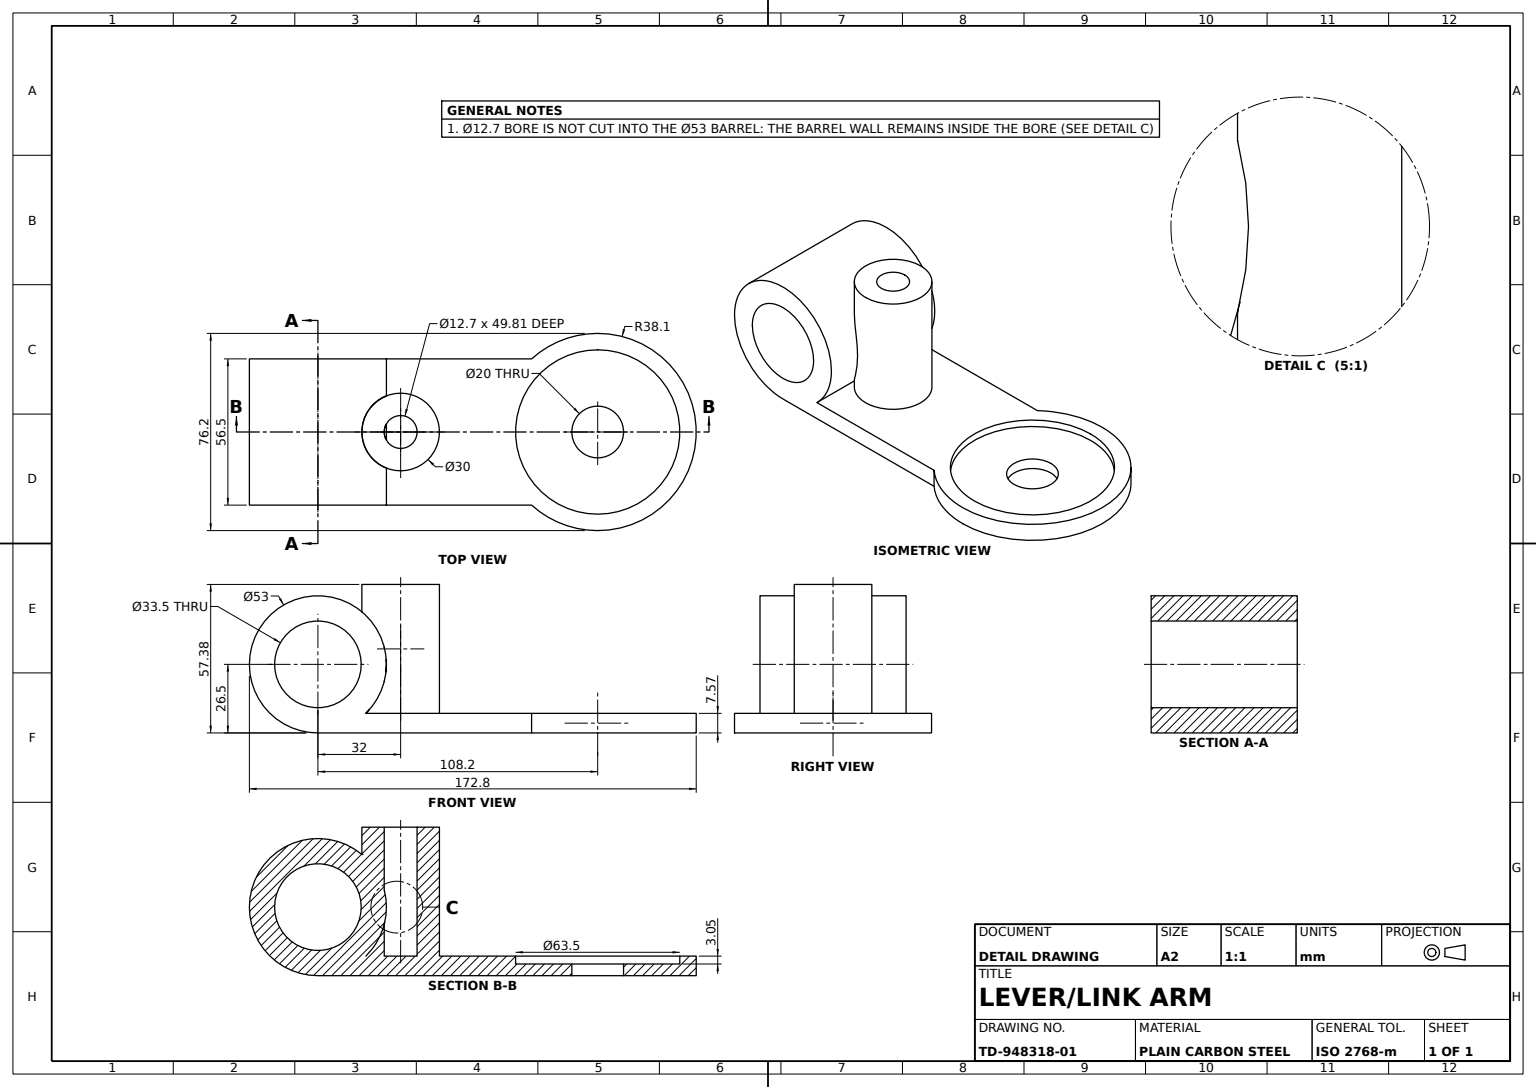
SolidWorks part; units mm, degrees
material "Plain Carbon Steel"
ref_plane "Front Plane" through (0, 0, 0) normal (0, 0, 1) x (1, 0, 0)
ref_plane "Top Plane" through (0, 0, 0) normal (0, 1, 0) x (1, 0, 0)
ref_plane "Right Plane" through (0, 0, 0) normal (1, 0, 0) x (0, 0, -1)
sketch "Pivot Tube Sketch" plane through (0, 0, 0) normal (0, 0, 1) x (1, 0, 0)
  circle A0 centre (0, 0) radius 26.5
  circle A1 centre (0, 0) radius 16.75
  dimension "D1" = 53
  dimension "D2" = 33.5
extrude "Pivot Tube Ø53xØ33.5" add sketch "Pivot Tube Sketch" along normal mid plane 56.5
sketch "Arm Profile Sketch" plane through (0, 0, 0) normal (0, 0, 1) x (1, 0, 0)
  line L1 (0, -26.5) -> (108.2, -26.5)
  line L2 (108.2, -26.5) -> (108.2, -18.935)
  line L3 (108.2, -18.935) -> (18.5396, -18.935)
  circle A0 centre (0, 0) radius 26.5 construction
  arc A1 (0, -26.5) -> (18.5396, -18.935) centre (0, 0) ccw
  dimension "D1" = 89.6604
  dimension "D2" = 108.2
  dimension "D3" = 7.565
extrude "Arm Plate" add sketch "Arm Profile Sketch" against normal mid plane 56.5
sketch "Post Sketch" plane through (0, 0, 0) normal (0, 1, 0) x (1, 0, 0)
  line L0 (108.2, 28.25) -> (108.2, -28.25) construction
  circle A0 centre (108.2, 0) radius 38.1
  circle A1 centre (108.2, 0) radius 31.75
  dimension "D1" = 63.5
  dimension "D2" = 76.2
extrude "Post Boss" add sketch "Post Sketch" against normal blind 26.5
sketch "Post Trim Sketch" plane through (0, 0, 0) normal (0, 0, 1) x (1, 0, 0)
  line L0 (70.1, 0) -> (146.3, 0)
  line L1 (146.3, 0) -> (146.3, -18.935)
  line L2 (146.3, -26.5) -> (146.3, 0) construction
  line L3 (146.3, -18.935) -> (70.1, -18.935)
  line L4 (70.1, -18.935) -> (70.1, 0)
extrude "Post Trim Cut" cut sketch "Post Trim Sketch" against normal mid plane 100
sketch "Mounting Pad Sketch" plane through (0, -18.935, 0) normal (0, 1, 0) x (1, 0, 0)
  line L0 (108.2, 28.25) -> (108.2, -28.25) construction
  circle A0 centre (108.2, 0) radius 31.75
  dimension "D1" = 63.5
extrude "Mounting Pad" add sketch "Mounting Pad Sketch" against normal blind 7.565
sketch "Pad Recess Sketch" plane through (0, -18.935, 0) normal (0, 1, 0) x (1, 0, 0)
  circle A0 centre (108.2, 0) radius 31.75
  dimension "D1" = 63.5
extrude "Pad Recess" cut sketch "Pad Recess Sketch" against normal blind 3.05
sketch "Pad Hole Sketch" plane through (0, -21.985, 0) normal (0, 1, 0) x (1, 0, 0)
  circle A0 centre (108.2, 0) radius 10
  dimension "D1" = 20
extrude "Pad Hole Ø20" cut sketch "Pad Hole Sketch" against normal through all
sketch "Arm Link Sketch" plane through (0, -18.935, 0) normal (0, 1, 0) x (1, 0, 0)
  line L0 (0, 0) -> (32, 0) construction
  circle A0 centre (32, 0) radius 15
  circle A1 centre (32, 0) radius 6.35
  dimension "D1" = 32
  dimension "D2" = 30
  dimension "D3" = 12.7
extrude "Arm Link Boss" add sketch "Arm Link Sketch" along normal blind 49.815
